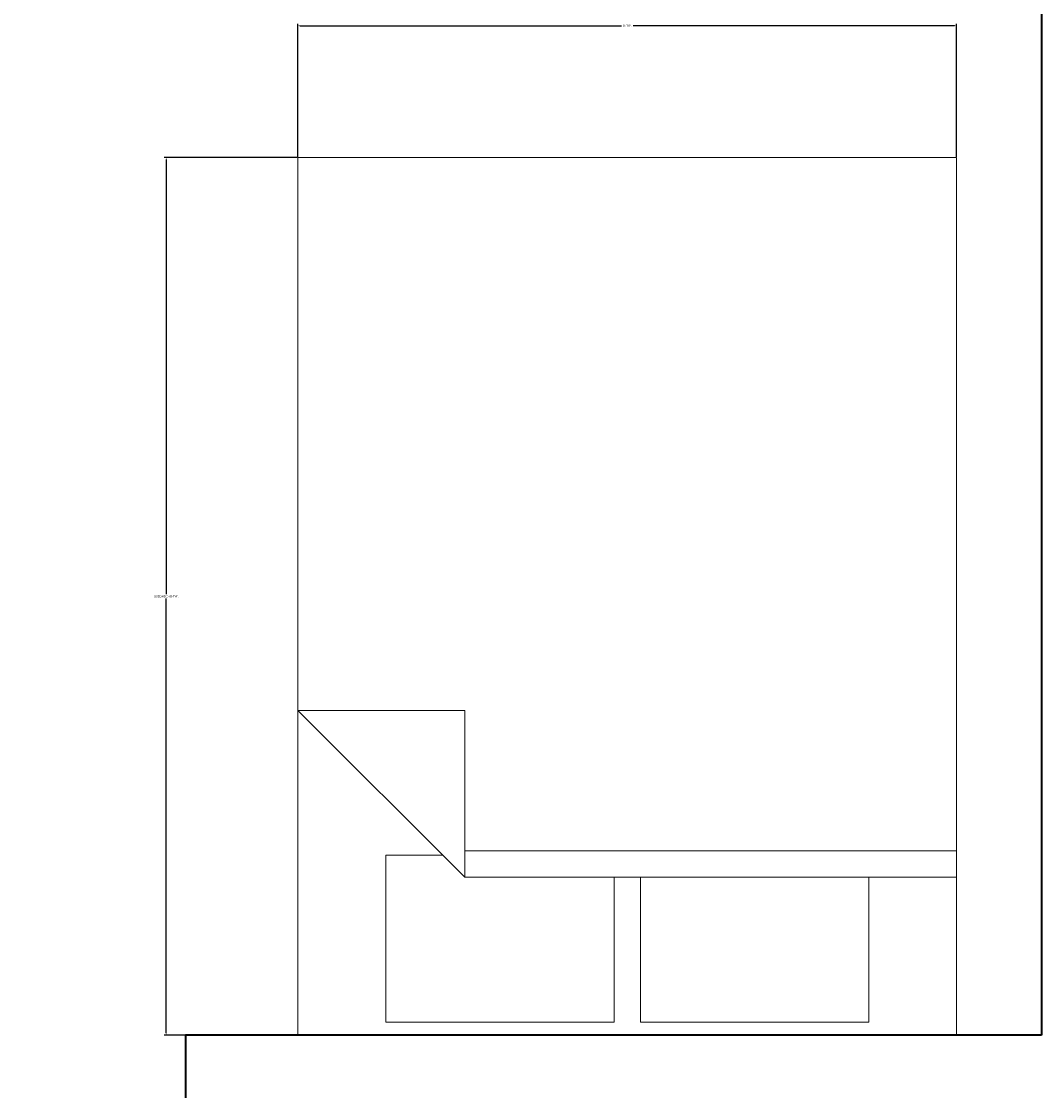
# Model space of a CAD drawing. Units: inches. Extents: x 4159 to 4826, y 299 to 1026.
# Tile 8 of 37: x 4354 to 4447, y 396 to 494. Entities that reach past the tile are written whole.
import ezdxf

# ---------------------------------------------------------------- set-up
doc = ezdxf.new("R2010")
doc.units = ezdxf.units.IN
for name, color, linetype, lineweight in [('A-ANNO-DIMS', 2, 'Continuous', 18), ('A-FURN', 8, 'Continuous', 18), ('A-WALL', 7, 'Continuous', 35)]:
    doc.layers.add(name, color=color, linetype=linetype, lineweight=lineweight)
doc.styles.get("Standard").update_dxf_attribs({"font": 'arial.ttf'})
doc.dimstyles.get("Standard").update_dxf_attribs({"dimtxt": 0.18, "dimasz": 0.18, "dimexe": 0.18, "dimexo": 0.0625, "dimgap": 0.09, "dimtad": 0, "dimtih": 1, "dimtoh": 1, "dimdec": 4, "dimzin": 0, "dimdsep": 46, "dimtxsty": 'Standard', "dimcen": 0.09, "dimadec": 0, "dimazin": 0, "dimtfac": 1, "dimtdec": 4, "dimtofl": 0, "dimtmove": 0, "dimatfit": 3, "dimfxl": 1, "dimtolj": 1, "dimtzin": 0, "dimarcsym": 0})

# ---------------------------------------------------------------- blocks, each defined once
blk = doc.blocks.new('Bed - Queen')
for p, q in [((0, -80.00003), (0, 0)), ((0, 0), (59.99999, 0)), ((59.99999, 0), (59.99999, -80.00003)), ((7.99999, -1.2), (28.79998, -1.2)), ((7.99999, -14.4), (7.99999, -1.2)), ((28.79998, -1.2), (28.79998, -14.4)), ((31.19999, -1.2), (51.99999, -1.2)), ((31.19999, -14.4), (31.19999, -1.2)), ((51.99999, -1.2), (51.99999, -16.4)), ((0, -14.4), (44.8, -14.4)), ((59.99999, -29.6), (44.8, -14.4)), ((44.8, -14.4), (44.8, -29.6)), ((51.99999, -16.4), (46.79936, -16.4)), ((44.8, -16.8), (0, -16.8)), ((44.8, -29.6), (59.99999, -29.6)), ((59.99999, -80.00003), (0, -80.00003))]:
    blk.add_line(p, q)
blk = doc.blocks.new('*D23')
at = {"layer": 'A-ANNO-DIMS', "color": 0, "lineweight": -2, "transparency": 16777216}
for p, q in [((4379.499, 481.254), (4367.382, 481.254)), ((4367.562, 481.074), (4367.562, 441.443)), ((4367.562, 401.434), (4367.562, 441.066)), ((4379.499, 401.254), (4367.382, 401.254))]:
    blk.add_line(p, q, dxfattribs=at)
at = {"layer": 'A-ANNO-DIMS', "color": 0, "transparency": 16777216}
for points in [[(4367.532, 481.074), (4367.592, 481.074), (4367.562, 481.254)], [(4367.532, 401.434), (4367.592, 401.434), (4367.562, 401.254)]]:
    blk.add_solid(points, dxfattribs=at)
at = {"layer": 'Defpoints', "color": 0, "transparency": 16777216}
for p in [(4379.562, 481.254), (4367.562, 401.254), (4379.562, 401.254)]:
    blk.add_point(p, dxfattribs=at)
at = {"layer": 'A-ANNO-DIMS', "color": 0, "transparency": 16777216, "insert": (4367.562, 441.254), "char_height": 0.18, "attachment_point": 5}
blk.add_mtext('\\A1;QUEEN BED 80 TYP.', dxfattribs=at)
blk = doc.blocks.new('*D24')
at = {"layer": 'A-ANNO-DIMS', "color": 0, "lineweight": -2, "transparency": 16777216}
for p, q in [((4379.562, 481.317), (4379.562, 493.434)), ((4379.742, 493.254), (4409.033, 493.254)), ((4439.382, 493.254), (4410.09, 493.254)), ((4439.562, 481.317), (4439.562, 493.434))]:
    blk.add_line(p, q, dxfattribs=at)
at = {"layer": 'A-ANNO-DIMS', "color": 0, "transparency": 16777216}
for points in [[(4379.742, 493.284), (4379.742, 493.224), (4379.562, 493.254)], [(4439.382, 493.284), (4439.382, 493.224), (4439.562, 493.254)]]:
    blk.add_solid(points, dxfattribs=at)
at = {"layer": 'Defpoints', "color": 0, "transparency": 16777216}
for p in [(4379.562, 493.254), (4379.562, 481.254), (4439.562, 481.254)]:
    blk.add_point(p, dxfattribs=at)
at = {"layer": 'A-ANNO-DIMS', "color": 0, "transparency": 16777216, "insert": (4409.562, 493.254), "char_height": 0.18, "attachment_point": 5}
blk.add_mtext('\\A1;60 TYP.', dxfattribs=at)
blk = doc.blocks.new('*D44')
at = {"layer": 'A-ANNO-DIMS', "color": 0, "lineweight": -2, "transparency": 16777216}
for p, q in [((4287.263, 963.093), (4158.88, 963.093)), ((4159.06, 962.913), (4159.06, 647.826)), ((4159.06, 332.375), (4159.06, 647.462)), ((4447.248, 332.195), (4158.88, 332.195))]:
    blk.add_line(p, q, dxfattribs=at)
at = {"layer": 'A-ANNO-DIMS', "color": 0, "transparency": 16777216}
for points in [[(4159.03, 962.913), (4159.09, 962.913), (4159.06, 963.093)], [(4159.03, 332.375), (4159.09, 332.375), (4159.06, 332.195)]]:
    blk.add_solid(points, dxfattribs=at)
at = {"layer": 'Defpoints', "color": 0, "transparency": 16777216}
for p in [(4287.326, 963.093), (4159.06, 332.195), (4447.31, 332.195)]:
    blk.add_point(p, dxfattribs=at)
at = {"layer": 'A-ANNO-DIMS', "color": 0, "transparency": 16777216, "insert": (4159.06, 647.644), "char_height": 0.18, "attachment_point": 5}
blk.add_mtext('\\A1;630.9', dxfattribs=at)

msp = doc.modelspace()

# ---------------------------------------------------------------- linework, layer by layer
at = {"layer": 'A-WALL'}
for p, q in [((4447.31, 533.254), (4447.31, 401.254)), ((4447.31, 401.254), (4369.31, 401.254)), ((4369.31, 401.254), (4369.31, 392.254))]:
    msp.add_line(p, q, dxfattribs=at)

# ---------------------------------------------------------------- block references
at = {"layer": 'A-FURN', "rotation": 180}
msp.add_blockref('Bed - Queen', (4439.562, 401.254), dxfattribs=at)

# ---------------------------------------------------------------- dimensions: what is measured, and where the dimension line sits
at = {"layer": 'A-ANNO-DIMS'}
dim = msp.add_linear_dim(base=(4159.06, 332.195), p1=(4287.326, 963.093), p2=(4447.31, 332.195), angle=90, dimstyle='Standard', override={"dimdec": 1, "dimlfac": 1, "dimrnd": 0, "dimzin": 0, "dimdsep": 46, "dimlunit": 2}, dxfattribs=at)
dim.commit()
dim.dimension.update_dxf_attribs({"geometry": '*D44', "text_midpoint": (4159.06, 647.644)})
for base, p1, p2, angle, text, picture, middle in [((4379.562, 493.254), (4439.562, 481.254), (4379.562, 481.254), 180, '<> TYP.', '*D24', (4409.562, 493.254)), ((4367.562, 401.254), (4379.562, 481.254), (4379.562, 401.254), 270, 'QUEEN BED <> TYP.', '*D23', (4367.562, 441.254))]:
    dim = msp.add_linear_dim(base=base, p1=p1, p2=p2, angle=angle, text=text, dimstyle='Standard', override={"dimdec": 0, "dimlfac": 1, "dimrnd": 0, "dimzin": 0, "dimdsep": 46, "dimlunit": 2}, dxfattribs=at)
    dim.commit()
    dim.dimension.update_dxf_attribs({"geometry": picture, "text_midpoint": middle})

doc.saveas('drawing.dxf')
